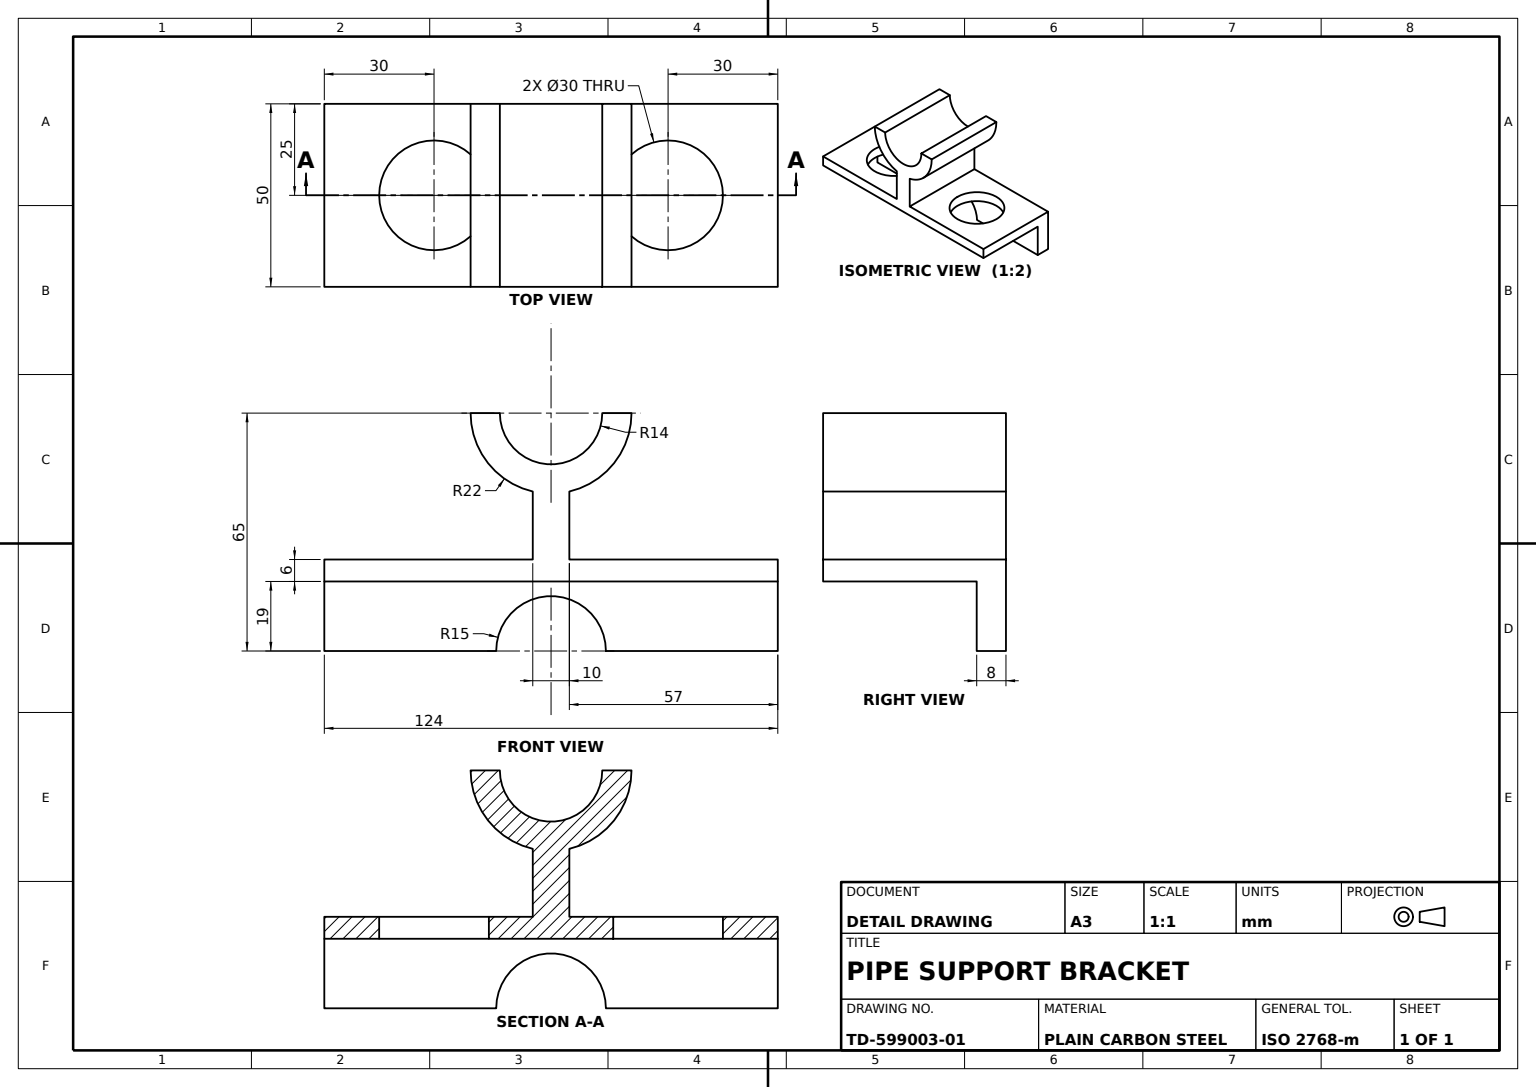
from build123d import *

# Parameters (mm, degrees)
BASE_ANGLE_DEPTH           = 124
SADDLE_BOSS_DEPTH          = 50
SADDLE_SEAT_CUT_DEPTH      = 50
RELIEF_CUT_DEPTH           = 50
MOUNTING_HOLES_SKETCH_R    = 15
MOUNTING_HOLES_2X_30_DEPTH = 20


with BuildPart() as part:
    # Base Angle Profile Sketch → Base Angle (new body)
    with BuildSketch(Plane.XY):
        Polygon((0, 0), (0, 25), (50, 25), (50, 19), (8, 19), (8, 0), align=None)
    extrude(amount=BASE_ANGLE_DEPTH)

    # Saddle Boss Sketch → Saddle Boss (add)
    with BuildSketch(Plane.ZY):
        with BuildLine():
            Line((84, 65), (62, 65))
            Line((62, 65), (40, 65))
            ThreePointArc((40, 65), (44.76631206, 51.325205669), (57, 43.575714714))
            Line((57, 43.575714714), (57, 25))
            Line((57, 25), (67, 25))
            Line((67, 25), (67, 43.575714714))
            ThreePointArc((67, 43.575714714), (79.23368794, 51.325205669), (84, 65))
        make_face()
    extrude(amount=-SADDLE_BOSS_DEPTH)

    # Saddle Seat Sketch → Saddle Seat Cut (cut)
    with BuildSketch(Plane.ZY):
        with BuildLine():
            Line((48, 65), (76, 65))
            ThreePointArc((76, 65), (62, 51), (48, 65))
        make_face()
    extrude(amount=-SADDLE_SEAT_CUT_DEPTH, mode=Mode.SUBTRACT)

    # Relief Cut Sketch → Relief Cut (cut)
    with BuildSketch(Plane.ZY):
        with BuildLine():
            Line((47, 0), (77, 0))
            ThreePointArc((77, 0), (62, 15), (47, 0))
        make_face()
    extrude(amount=-RELIEF_CUT_DEPTH, mode=Mode.SUBTRACT)

    # Mounting Holes Sketch → Mounting Holes 2xØ30 (cut)
    with BuildSketch(Plane.XZ.offset(-19)):
        with Locations(Location((25, 94, 0), (0, 0, 270))):
            Circle(MOUNTING_HOLES_SKETCH_R)
        with Locations(Location((25, 30, 0), (0, 0, 270))):
            Circle(MOUNTING_HOLES_SKETCH_R)
    extrude(amount=-MOUNTING_HOLES_2X_30_DEPTH, mode=Mode.SUBTRACT)


solid = part.part
